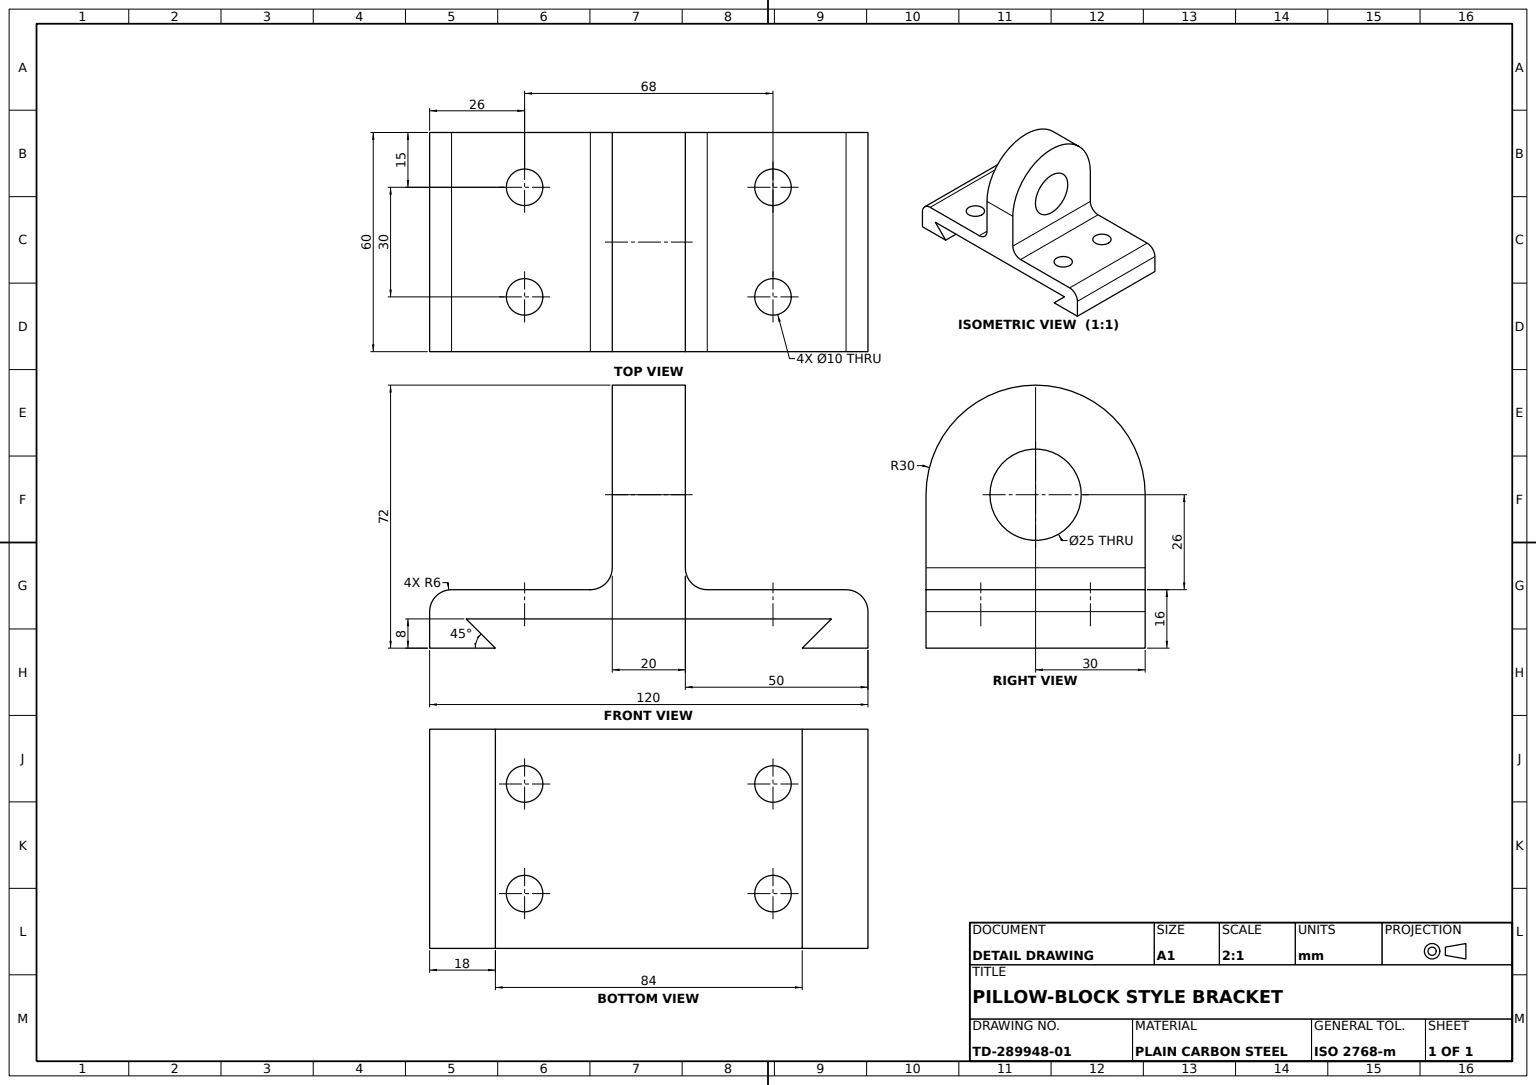
from build123d import *

# Parameters (mm, degrees)
BASE_PLATE_DEPTH         = 60
MOUNTING_HOLES_SKETCH_R  = 5
MOUNTING_HOLES_DEPTH     = 60
EYE_UPRIGHT_PROFILE_R    = 12.5
EYE_UPRIGHT_DEPTH        = 10
UPRIGHT_ROOT_FILLET_R6_R = 6


with BuildPart() as part:
    # Base Plate Profile → Base Plate (new body)
    with BuildSketch(Plane.XY):
        Polygon((0, 0), (50, 0), (42, -8), (60, -8), (60, 8), (-60, 8), (-60, -8), (-42, -8), (-50, 0), align=None)
    extrude(amount=-BASE_PLATE_DEPTH)

    # Mounting Holes Sketch → Mounting Holes (cut)
    with BuildSketch(Plane(origin=(0, 8, 0), x_dir=(1, 0, 0), z_dir=(0, 1, 0))):
        with Locations(Location((34, 45, 0), (0, 0, 180))):
            Circle(MOUNTING_HOLES_SKETCH_R)
        with Locations(Location((34, 15, 0), (0, 0, 180))):
            Circle(MOUNTING_HOLES_SKETCH_R)
        with Locations(Location((-34, 45, 0), (0, 0, 180))):
            Circle(MOUNTING_HOLES_SKETCH_R)
        with Locations(Location((-34, 15, 0), (0, 0, 180))):
            Circle(MOUNTING_HOLES_SKETCH_R)
    extrude(amount=-MOUNTING_HOLES_DEPTH, mode=Mode.SUBTRACT)

    # Eye Upright Profile → Eye Upright (add, symmetric)
    with BuildSketch(Plane(origin=(0, 0, 0), x_dir=(0, 0, -1), z_dir=(1, 0, 0))):
        with BuildLine():
            Line((0, 8), (0, 34))
            ThreePointArc((0, 34), (30, 64), (60, 34))
            Line((60, 34), (60, 8))
            Line((60, 8), (0, 8))
        make_face()
        with Locations((30, 34)):
            Circle(EYE_UPRIGHT_PROFILE_R, mode=Mode.SUBTRACT)
    extrude(amount=EYE_UPRIGHT_DEPTH, both=True)

    # Upright Root Fillet R6
    upright_root_fillet_r6_edges = [part.edges().sort_by_distance(p)[0] for p in [
        (-60, 8, -30),
        (60, 8, -30),
        (10, 8, -30),
        (-10, 8, -30),
    ]]
    fillet(upright_root_fillet_r6_edges, radius=UPRIGHT_ROOT_FILLET_R6_R)


solid = part.part
